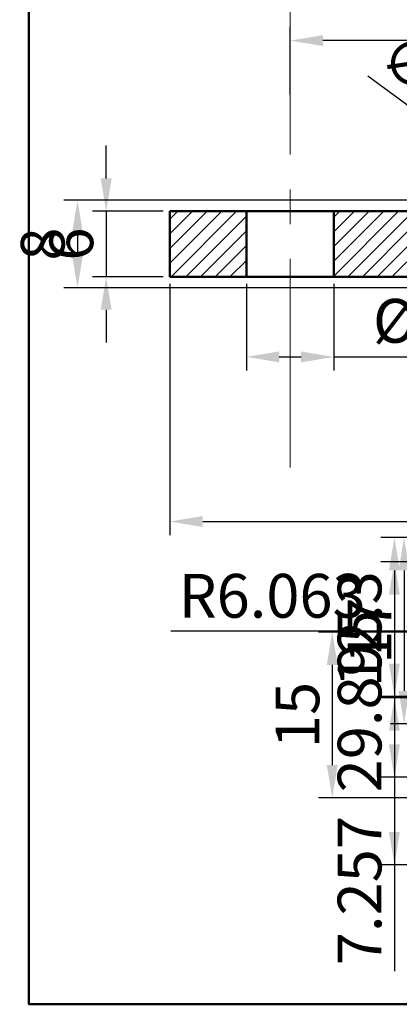
# Model space of a CAD drawing. Units: millimetres. Extents: x 139 to 291, y 28 to 164.
# Tile 1 of 5: x 139 to 174, y 28 to 118. Entities that reach past the tile are written whole.
import ezdxf

# ---------------------------------------------------------------- set-up
doc = ezdxf.new("R2010")
doc.units = ezdxf.units.MM
doc.linetypes.add('CENTER2', pattern=[28.575, 19.05, -3.175, 3.175, -3.175])
for name, color, linetype, lineweight in [('M-CNTR', 1, 'CENTER2', 18), ('M-DIMS', 2, 'Continuous', 25), ('M-HATC', 8, 'Continuous', 18), ('M-OUTL', 7, 'Continuous', 50)]:
    doc.layers.add(name, color=color, linetype=linetype, lineweight=lineweight)
doc.styles.get("Standard").update_dxf_attribs({"font": 'arial.ttf'})
doc.dimstyles.new('ISO-25', dxfattribs={"dimtxt": 4, "dimasz": 3, "dimexe": 1.25, "dimexo": 0.625, "dimtad": 1, "dimdec": 0, "dimtxsty": 'Standard', "dimcen": 2.5, "dimadec": 0, "dimazin": 0, "dimtfac": 1, "dimtdec": 0, "dimtmove": 0, "dimatfit": 3, "dimfxl": 1, "dimarcsym": 0})

# ---------------------------------------------------------------- blocks, each defined once
blk = doc.blocks.new('*U1')
at = {"layer": 'M-CNTR', "color": 0, "transparency": 16777216}
for p, q in [((0, 2.2), (0, 14.5)), ((-14.5, 0), (-2.2, 0)), ((2.2, 0), (65.925, 0)), ((0, -57.955), (0, -2.2))]:
    blk.add_line(p, q, dxfattribs=at)
at = {"layer": 'M-CNTR', "color": 0, "linetype": 'Continuous', "transparency": 16777216}
for p, q in [((0, -1.1), (0, 1.1)), ((-1.1, 0), (1.1, 0))]:
    blk.add_line(p, q, dxfattribs=at)
blk = doc.blocks.new('*D6')
at = {"layer": 'Defpoints', "color": 0, "transparency": 16777216}
for p in [(163.636, 116.256), (163.636, 110.703), (201.636, 110.703)]:
    blk.add_point(p, dxfattribs=at)
at = {"layer": 'M-DIMS', "color": 0, "lineweight": -2, "transparency": 16777216}
for p, q in [((163.636, 111.328), (163.636, 117.506)), ((201.636, 111.328), (201.636, 117.506)), ((198.636, 116.256), (166.636, 116.256))]:
    blk.add_line(p, q, dxfattribs=at)
at = {"layer": 'M-DIMS', "color": 0, "transparency": 16777216}
for points in [[(166.636, 116.756), (166.636, 115.756), (163.636, 116.256)], [(198.636, 116.756), (198.636, 115.756), (201.636, 116.256)]]:
    blk.add_solid(points, dxfattribs=at)
at = {"layer": 'M-DIMS', "color": 0, "transparency": 16777216, "insert": (182.636, 118.925), "char_height": 4, "attachment_point": 5}
blk.add_mtext('38', dxfattribs=at)
blk = doc.blocks.new('*D11')
at = {"layer": 'Defpoints', "color": 0, "transparency": 16777216}
for p in [(159.636, 94.663), (167.636, 94.663), (167.636, 87.351)]:
    blk.add_point(p, dxfattribs=at)
at = {"layer": 'M-DIMS', "color": 0, "lineweight": -2, "transparency": 16777216}
for p, q in [((159.636, 94.038), (159.636, 86.101)), ((167.636, 94.038), (167.636, 86.101)), ((162.636, 87.351), (164.636, 87.351)), ((167.636, 87.351), (178.868, 87.351))]:
    blk.add_line(p, q, dxfattribs=at)
at = {"layer": 'M-DIMS', "color": 0, "transparency": 16777216}
for points in [[(162.636, 87.851), (162.636, 86.851), (159.636, 87.351)], [(164.636, 87.851), (164.636, 86.851), (167.636, 87.351)]]:
    blk.add_solid(points, dxfattribs=at)
at = {"layer": 'M-DIMS', "color": 0, "transparency": 16777216, "insert": (174.752, 90.13), "char_height": 4, "attachment_point": 5}
blk.add_mtext('%%C8', dxfattribs=at)
blk = doc.blocks.new('*D13')
at = {"layer": 'Defpoints', "color": 0, "transparency": 16777216}
for p in [(152.636, 100.663), (146.807, 94.663), (152.636, 94.663)]:
    blk.add_point(p, dxfattribs=at)
at = {"layer": 'M-DIMS', "color": 0, "lineweight": -2, "transparency": 16777216}
for p, q in [((146.807, 103.663), (146.807, 106.663)), ((152.011, 100.663), (145.557, 100.663)), ((146.807, 100.663), (146.807, 94.663)), ((152.011, 94.663), (145.557, 94.663)), ((146.807, 91.663), (146.807, 88.663))]:
    blk.add_line(p, q, dxfattribs=at)
at = {"layer": 'M-DIMS', "color": 0, "transparency": 16777216}
for points in [[(146.307, 103.663), (147.307, 103.663), (146.807, 100.663)], [(146.307, 91.663), (147.307, 91.663), (146.807, 94.663)]]:
    blk.add_solid(points, dxfattribs=at)
at = {"layer": 'M-DIMS', "color": 0, "transparency": 16777216, "insert": (144.14, 97.663), "char_height": 4, "attachment_point": 5, "rotation": 90}
blk.add_mtext('6', dxfattribs=at)
blk = doc.blocks.new('*D27')
at = {"layer": 'Defpoints', "color": 0, "transparency": 16777216}
for p in [(180.776, 70.836), (174.061, 53.836), (180.776, 53.836)]:
    blk.add_point(p, dxfattribs=at)
at = {"layer": 'M-DIMS', "color": 0, "lineweight": -2, "transparency": 16777216}
for p, q in [((180.151, 70.836), (172.811, 70.836)), ((174.061, 67.836), (174.061, 56.836)), ((180.151, 53.836), (172.811, 53.836))]:
    blk.add_line(p, q, dxfattribs=at)
at = {"layer": 'M-DIMS', "color": 0, "transparency": 16777216}
for points in [[(173.561, 67.836), (174.561, 67.836), (174.061, 70.836)], [(173.561, 56.836), (174.561, 56.836), (174.061, 53.836)]]:
    blk.add_solid(points, dxfattribs=at)
at = {"layer": 'M-DIMS', "color": 0, "transparency": 16777216, "insert": (171.428, 62.336), "char_height": 4, "attachment_point": 5, "rotation": 90}
blk.add_mtext('17', dxfattribs=at)
blk = doc.blocks.new('*D28')
at = {"layer": 'Defpoints', "color": 0, "transparency": 16777216}
for p in [(177.287, 62.199), (167.49, 47.061), (196.787, 47.061)]:
    blk.add_point(p, dxfattribs=at)
at = {"layer": 'M-DIMS', "color": 0, "lineweight": -2, "transparency": 16777216}
for p, q in [((176.662, 62.199), (166.24, 62.199)), ((167.49, 59.199), (167.49, 50.061)), ((196.162, 47.061), (166.24, 47.061))]:
    blk.add_line(p, q, dxfattribs=at)
at = {"layer": 'M-DIMS', "color": 0, "transparency": 16777216}
for points in [[(166.99, 59.199), (167.99, 59.199), (167.49, 62.199)], [(166.99, 50.061), (167.99, 50.061), (167.49, 47.061)]]:
    blk.add_solid(points, dxfattribs=at)
at = {"layer": 'M-DIMS', "color": 0, "transparency": 16777216, "insert": (164.822, 54.63), "char_height": 4, "attachment_point": 5, "rotation": 90}
blk.add_mtext('15', dxfattribs=at)
blk = doc.blocks.new('*D36')
at = {"layer": 'Defpoints', "color": 0, "transparency": 16777216}
for p in [(152.636, 94.663), (205.636, 89.163), (205.636, 72.308)]:
    blk.add_point(p, dxfattribs=at)
at = {"layer": 'M-DIMS', "color": 0, "lineweight": -2, "transparency": 16777216}
for p, q in [((152.636, 94.038), (152.636, 71.058)), ((205.636, 88.538), (205.636, 71.058)), ((155.636, 72.308), (202.636, 72.308))]:
    blk.add_line(p, q, dxfattribs=at)
at = {"layer": 'M-DIMS', "color": 0, "transparency": 16777216}
for points in [[(155.636, 72.808), (155.636, 71.808), (152.636, 72.308)], [(202.636, 72.808), (202.636, 71.808), (205.636, 72.308)]]:
    blk.add_solid(points, dxfattribs=at)
at = {"layer": 'M-DIMS', "color": 0, "transparency": 16777216, "insert": (179.136, 74.977), "char_height": 4, "attachment_point": 5}
blk.add_mtext('53', dxfattribs=at)
blk = doc.blocks.new('*D39')
at = {"layer": 'Defpoints', "color": 0, "transparency": 16777216}
for p in [(187.636, 101.663), (144.186, 93.663), (187.636, 93.663)]:
    blk.add_point(p, dxfattribs=at)
at = {"layer": 'M-DIMS', "color": 0, "lineweight": -2, "transparency": 16777216}
for p, q in [((187.011, 101.663), (142.936, 101.663)), ((144.186, 98.663), (144.186, 96.663)), ((187.011, 93.663), (142.936, 93.663))]:
    blk.add_line(p, q, dxfattribs=at)
at = {"layer": 'M-DIMS', "color": 0, "transparency": 16777216}
for points in [[(143.686, 98.663), (144.686, 98.663), (144.186, 101.663)], [(143.686, 96.663), (144.686, 96.663), (144.186, 93.663)]]:
    blk.add_solid(points, dxfattribs=at)
at = {"layer": 'M-DIMS', "color": 0, "transparency": 16777216, "insert": (141.519, 97.663), "char_height": 4, "attachment_point": 5, "rotation": 90}
blk.add_mtext('8', dxfattribs=at)
blk = doc.blocks.new('*D43')
at = {"layer": 'Defpoints', "color": 0, "transparency": 16777216}
for p in [(179.287, 70.836), (173.176, 40.942), (198.299, 40.942)]:
    blk.add_point(p, dxfattribs=at)
at = {"layer": 'M-DIMS', "color": 0, "lineweight": -2, "transparency": 16777216}
for p, q in [((178.662, 70.836), (171.926, 70.836)), ((173.176, 67.836), (173.176, 43.942)), ((197.674, 40.942), (171.926, 40.942))]:
    blk.add_line(p, q, dxfattribs=at)
at = {"layer": 'M-DIMS', "color": 0, "transparency": 16777216}
for points in [[(172.676, 67.836), (173.676, 67.836), (173.176, 70.836)], [(172.676, 43.942), (173.676, 43.942), (173.176, 40.942)]]:
    blk.add_solid(points, dxfattribs=at)
at = {"layer": 'M-DIMS', "color": 0, "transparency": 16777216, "insert": (170.509, 55.889), "char_height": 4, "attachment_point": 5, "rotation": 90}
blk.add_mtext('29.895', dxfattribs=at)
blk = doc.blocks.new('*D46')
at = {"layer": 'Defpoints', "color": 0, "transparency": 16777216}
for p in [(187.287, 68.624), (173.176, 56.324), (187.287, 56.324)]:
    blk.add_point(p, dxfattribs=at)
at = {"layer": 'M-DIMS', "color": 0, "lineweight": -2, "transparency": 16777216}
for p, q in [((186.662, 68.624), (171.926, 68.624)), ((173.176, 65.624), (173.176, 59.324)), ((186.662, 56.324), (171.926, 56.324))]:
    blk.add_line(p, q, dxfattribs=at)
at = {"layer": 'M-DIMS', "color": 0, "transparency": 16777216}
for points in [[(172.676, 65.624), (173.676, 65.624), (173.176, 68.624)], [(172.676, 59.324), (173.676, 59.324), (173.176, 56.324)]]:
    blk.add_solid(points, dxfattribs=at)
at = {"layer": 'M-DIMS', "color": 0, "transparency": 16777216, "insert": (170.507, 62.474), "char_height": 4, "attachment_point": 5, "rotation": 90}
blk.add_mtext('12.3', dxfattribs=at)
blk = doc.blocks.new('*D50')
at = {"layer": 'Defpoints', "color": 0, "transparency": 16777216}
for p in [(198.299, 56.199), (173.176, 48.942), (198.299, 48.942)]:
    blk.add_point(p, dxfattribs=at)
at = {"layer": 'M-DIMS', "color": 0, "lineweight": -2, "transparency": 16777216}
for p, q in [((197.674, 56.199), (171.926, 56.199)), ((173.176, 53.199), (173.176, 51.942)), ((197.674, 48.942), (171.926, 48.942)), ((173.176, 48.942), (173.176, 31.227))]:
    blk.add_line(p, q, dxfattribs=at)
at = {"layer": 'M-DIMS', "color": 0, "transparency": 16777216}
for points in [[(172.676, 53.199), (173.676, 53.199), (173.176, 56.199)], [(172.676, 51.942), (173.676, 51.942), (173.176, 48.942)]]:
    blk.add_solid(points, dxfattribs=at)
at = {"layer": 'M-DIMS', "color": 0, "transparency": 16777216, "insert": (170.509, 38.584), "char_height": 4, "attachment_point": 5, "rotation": 90}
blk.add_mtext('7.257', dxfattribs=at)
blk = doc.blocks.new('*D57')
at = {"layer": 'Defpoints', "color": 0, "transparency": 16777216}
for p in [(184.675, 102.725), (198.332, 92.602)]:
    blk.add_point(p, dxfattribs=at)
at = {"layer": 'M-DIMS', "color": 0, "lineweight": -2, "transparency": 16777216}
for p, q in [((170.751, 113.046), (182.265, 104.511)), ((198.332, 92.602), (184.675, 102.725)), ((200.743, 90.815), (203.153, 89.029))]:
    blk.add_line(p, q, dxfattribs=at)
at = {"layer": 'M-DIMS', "color": 0, "transparency": 16777216}
for points in [[(182.563, 104.913), (181.967, 104.11), (184.675, 102.725)], [(201.04, 91.217), (200.445, 90.414), (198.332, 92.602)]]:
    blk.add_solid(points, dxfattribs=at)
at = {"layer": 'M-DIMS', "color": 0, "transparency": 16777216, "insert": (176.958, 111.904), "char_height": 4, "attachment_point": 5, "rotation": 323.45299}
blk.add_mtext('∅17', dxfattribs=at)
blk = doc.blocks.new('*D60')
at = {"layer": 'Defpoints', "color": 0, "transparency": 16777216}
for p in [(177.287, 62.336), (183.35, 62.336)]:
    blk.add_point(p, dxfattribs=at)
at = {"layer": 'M-DIMS', "color": 0, "lineweight": -2, "transparency": 16777216}
for p, q in [((152.711, 62.334), (174.287, 62.336)), ((183.35, 62.336), (177.287, 62.336))]:
    blk.add_line(p, q, dxfattribs=at)
at = {"layer": 'M-DIMS', "color": 0, "transparency": 16777216}
blk.add_solid([(174.287, 62.836), (174.287, 61.836), (177.287, 62.336)], dxfattribs=at)
at = {"layer": 'M-DIMS', "color": 0, "transparency": 16777216, "insert": (161.999, 65.004), "char_height": 4, "attachment_point": 5, "rotation": 0.00419}
blk.add_mtext('R6.063', dxfattribs=at)

msp = doc.modelspace()

# ---------------------------------------------------------------- hatches: boundary and pattern name
at = {"layer": 'M-HATC'}
h = msp.add_hatch(dxfattribs=at)
h.set_pattern_fill('ANSI31', color=256, scale=0.3)
h.set_pattern_definition([(45, (0, -8.2379), (-0.6735192, 0.6735192), [])])
h.paths.add_polyline_path([(174.6359, 99.1632), (174.6359, 100.6632), (167.6359, 100.6632), (167.6359, 94.6632), (174.6359, 94.6632), (174.6359, 96.1632), (183.1373, 96.1632, 0.2343961), (187.6359, 90.0943), (191.6359, 90.6632), (191.6359, 91.1632), (201.6359, 91.1632), (201.6359, 93.1632), (187.6359, 93.6632), (183.6359, 97.6632), (187.6359, 101.6632), (201.6359, 102.1632), (201.6359, 104.1632), (191.6359, 104.1632), (191.6359, 104.6632), (187.6359, 105.2322, 0.2343961), (183.1373, 99.1632)])
h.paths.add_polyline_path([(159.6359, 94.6632), (159.6359, 100.6632), (152.6359, 100.6632), (152.6359, 94.6632)])

# ---------------------------------------------------------------- linework, layer by layer
at = {"layer": 'M-OUTL'}
for p, q in [((152.6359, 100.6632), (163.6359, 100.6632)), ((152.6359, 100.6632), (152.6359, 94.6632)), ((159.6359, 100.6632), (159.6359, 94.6632)), ((163.6359, 100.6632), (174.6359, 100.6632)), ((167.6359, 100.6632), (167.6359, 94.6632)), ((174.6359, 94.6632), (152.6359, 94.6632))]:
    msp.add_line(p, q, dxfattribs=at)
msp.add_lwpolyline([(139.74, 164.2339), (291.244, 164.2339), (291.244, 28.1944), (139.74, 28.1944)], close=True, dxfattribs=at)

# ---------------------------------------------------------------- block references
at = {"layer": 'M-CNTR'}
msp.add_blockref('*U1', (163.6359, 135.2132), dxfattribs=at)

# ---------------------------------------------------------------- dimensions: what is measured, and where the dimension line sits
at = {"layer": 'M-DIMS'}
for base, p1, p2, override, picture, middle in [((163.6359, 116.2564), (201.6359, 110.7027), (163.6359, 110.7027), {"dimclrd": 0, "dimclre": 0, "dimclrt": 0}, '*D6', (182.6359, 118.9251)), ((205.6359, 72.3085), (152.6359, 94.6632), (205.6359, 89.1632), {"dimdec": 0, "dimlfac": 1, "dimrnd": 0, "dimzin": 0, "dimdsep": 46, "dimlunit": 2}, '*D36', (179.1359, 74.9771))]:
    dim = msp.add_linear_dim(base=base, p1=p1, p2=p2, dimstyle='ISO-25', override=override, dxfattribs=at)
    dim.commit()
    dim.dimension.update_dxf_attribs({"geometry": picture, "text_midpoint": middle})
dim = msp.add_diameter_dim_2p(p1=(198.3325, 92.6016), p2=(184.6752, 102.7248), dimstyle='ISO-25', override={"dimdec": 0, "dimlfac": 1, "dimrnd": 0, "dimzin": 0, "dimdsep": 46, "dimlunit": 2}, dxfattribs=at)
dim.commit()
dim.dimension.update_dxf_attribs({"geometry": '*D57', "text_midpoint": (175.3032, 109.6717), "dimtype": 163})
for base, p1, p2, override, picture, middle in [((146.8072, 94.6632), (152.6359, 100.6632), (152.6359, 94.6632), {"dimclrd": 0, "dimclre": 0, "dimclrt": 0}, '*D13', (144.1399, 97.6632)), ((144.1859, 93.6632), (187.6359, 101.6632), (187.6359, 93.6632), {"dimdec": 0, "dimlfac": 1, "dimrnd": 0, "dimzin": 0, "dimdsep": 46, "dimlunit": 2}, '*D39', (141.5186, 97.6632)), ((173.1758, 40.9417), (179.2871, 70.8364), (198.2992, 40.9417), {"dimdec": 3, "dimlfac": 1, "dimrnd": 0, "dimzin": 0, "dimdsep": 46, "dimlunit": 2}, '*D43', (170.5086, 55.8891)), ((174.0612, 53.8364), (180.7759, 70.8364), (180.7759, 53.8364), {"dimclrd": 0, "dimclre": 0, "dimclrt": 0}, '*D27', (171.428, 62.3364)), ((173.1758, 56.3244), (187.2871, 68.6242), (187.2871, 56.3244), {"dimdec": 1, "dimlfac": 1, "dimrnd": 0, "dimzin": 0, "dimdsep": 46, "dimlunit": 2}, '*D46', (170.5072, 62.4743)), ((167.4897, 47.0608), (177.2871, 62.1986), (196.7871, 47.0608), {"dimclrd": 0, "dimclre": 0, "dimclrt": 0}, '*D28', (164.8224, 54.6297)), ((173.1758, 48.9417), (198.2992, 56.1986), (198.2992, 48.9417), {"dimdec": 3, "dimlfac": 1, "dimrnd": 0, "dimzin": 0, "dimdsep": 46, "dimlunit": 2}, '*D50', (170.5086, 38.5841))]:
    dim = msp.add_linear_dim(base=base, p1=p1, p2=p2, angle=90, dimstyle='ISO-25', override=override, dxfattribs=at)
    dim.commit()
    dim.dimension.update_dxf_attribs({"geometry": picture, "text_midpoint": middle})
dim = msp.add_linear_dim(base=(167.6359, 87.3506), p1=(159.6359, 94.6632), p2=(167.6359, 94.6632), text='%%C<>', dimstyle='ISO-25', override={"dimclrd": 0, "dimclre": 0, "dimclrt": 0}, dxfattribs=at)
dim.commit()
dim.dimension.update_dxf_attribs({"geometry": '*D11', "text_midpoint": (174.752, 90.1297)})
dim = msp.add_radius_dim(center=(183.3496, 62.3364), mpoint=(177.2871, 62.336), dimstyle='ISO-25', override={"dimdec": 3, "dimlfac": 1, "dimrnd": 0, "dimzin": 0, "dimdsep": 46, "dimlunit": 2}, dxfattribs=at)
dim.commit()
dim.dimension.update_dxf_attribs({"geometry": '*D60', "text_midpoint": (161.9989, 65.0035)})

doc.saveas('drawing.dxf')
